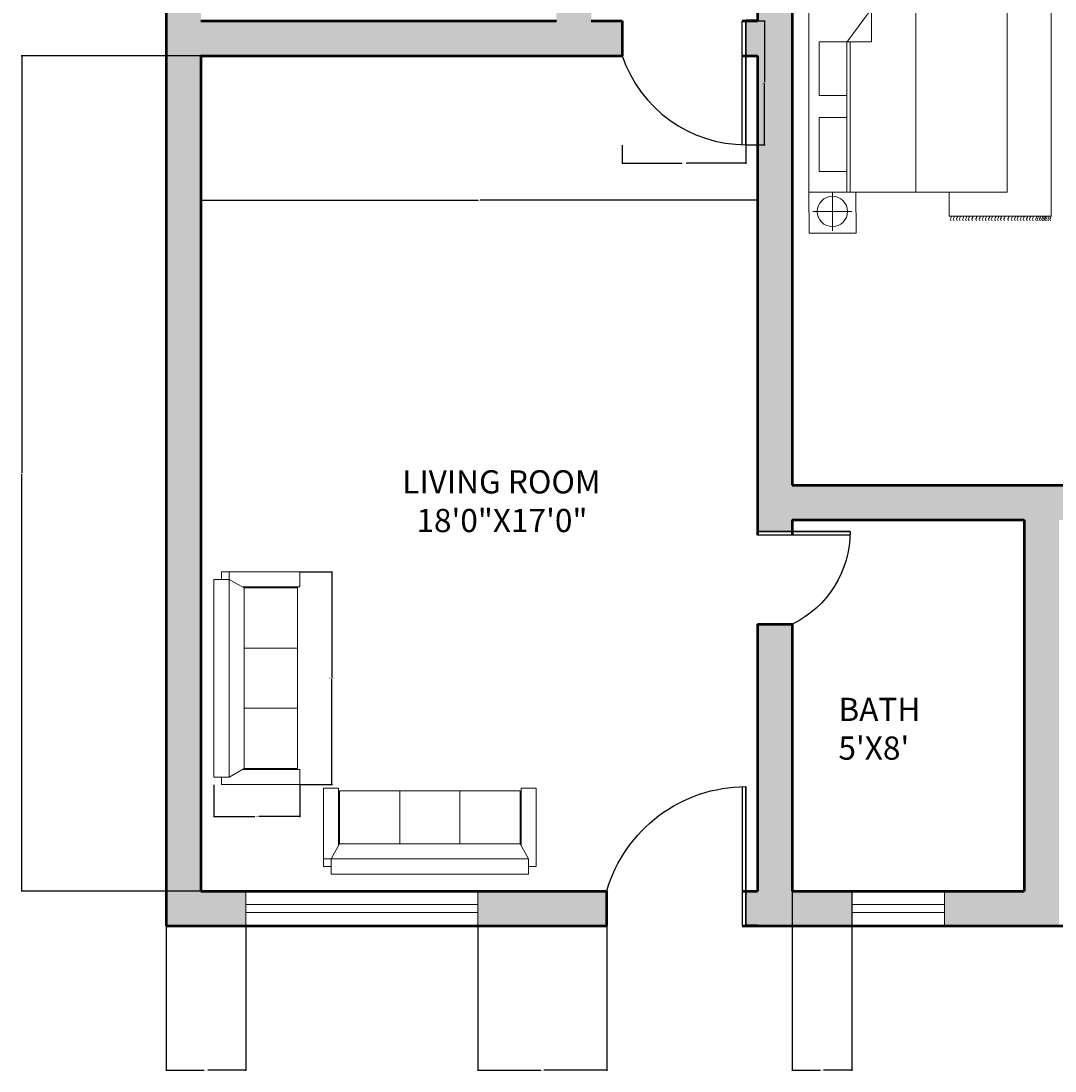
# Model space of a CAD drawing. Units: inches. Extents: x 383 to 970, y 275 to 1088.
# Tile 1 of 11: x 383 to 650, y 275 to 546. Entities that reach past the tile are written whole.
import ezdxf

# ---------------------------------------------------------------- set-up
doc = ezdxf.new("R2010")
doc.units = ezdxf.units.IN
doc.header["$MEASUREMENT"] = 0
for name, color, linetype, lineweight in [('A-ANNO-DIMS', 2, 'Continuous', 18), ('A-AREA-IDEN', 7, 'Continuous', 18), ('A-DOOR', 3, 'Continuous', 25), ('A-FURN', 8, 'Continuous', 18), ('A-GLAZ', 4, 'Continuous', 18), ('A-WALL', 7, 'Continuous', 50)]:
    doc.layers.add(name, color=color, linetype=linetype, lineweight=lineweight)
doc.layers.add('A-WALL-PATT', color=251, linetype='Continuous', lineweight=13, true_color=0x636466)
doc.styles.get("Standard").update_dxf_attribs({"font": 'arial.ttf'})
doc.dimstyles.get("Standard").update_dxf_attribs({"dimtxt": 0.18, "dimasz": 0.18, "dimexe": 0.18, "dimexo": 0.0625, "dimgap": 0.09, "dimtad": 0, "dimtih": 1, "dimtoh": 1, "dimdec": 4, "dimzin": 0, "dimdsep": 46, "dimtxsty": 'Standard', "dimcen": 0.09, "dimadec": 0, "dimazin": 0, "dimtfac": 1, "dimtdec": 4, "dimtofl": 0, "dimtmove": 0, "dimatfit": 3, "dimfxl": 1, "dimtolj": 1, "dimtzin": 0, "dimarcsym": 0})

# ---------------------------------------------------------------- blocks, each defined once
blk = doc.blocks.new('BED-DOUBLE-WITH-NIGHTSTANDS')
for p, q in [((6.09, 68.68), (6.09, 58.62)), ((36.42, 67.59), (62.78, 67.59)), ((36.42, 58.05), (36.42, 67.59)), ((62.78, 67.59), (62.78, 4.35)), ((1.07, 63.65), (11.12, 63.65)), ((9.97, 49.39), (16.32, 58)), ((16.32, 49.44), (16.32, 58)), ((27.82, 58.05), (27.82, 10.63)), ((9.97, 49.44), (16.32, 49.44)), ((9.97, 49.39), (9.97, 10.63)), ((10.78, 49.44), (10.78, 10.63)), ((6.2, 10.63), (6.2, 0.57)), ((36.42, 4.35), (36.42, 10.65)), ((1.17, 5.6), (11.22, 5.6)), ((62.78, 4.35), (36.42, 4.35))]:
    blk.add_line(p, q)
for points in [[(12.29, 58.05), (12.19, 68.68), (0, 68.68), (0.1, 58.05)], [(0.1, 58.05), (51.42, 58.05), (51.42, 10.63), (0.1, 10.63)], [(2.8, 49.44), (9.97, 49.44), (9.97, 35.55), (2.8, 35.55)], [(2.8, 29.88), (9.97, 29.88), (9.97, 15.98), (2.8, 15.98)], [(12.39, 0), (12.29, 10.63), (0.1, 10.63), (0.21, 0)]]:
    blk.add_lwpolyline(points, close=True)
for centre in [(6.09, 63.65), (6.2, 5.6)]:
    blk.add_circle(centre, 3.92)
for points, knots in [([(36.95, 68.71), (36.83, 68.61), (36.59, 68.42), (36.83, 68.08), (37, 67.8), (36.89, 67.65), (36.85, 67.58)], [0, 0, 0, 0, 0.400747, 0.791423, 1.067667, 1.29709, 1.29709, 1.29709, 1.29709]), ([(37.73, 68.71), (37.61, 68.61), (37.37, 68.42), (37.61, 68.08), (37.78, 67.8), (37.67, 67.65), (37.62, 67.58)], [0, 0, 0, 0, 0.400747, 0.791423, 1.067667, 1.29709, 1.29709, 1.29709, 1.29709]), ([(38.54, 68.71), (38.42, 68.61), (38.18, 68.42), (38.42, 68.08), (38.59, 67.8), (38.49, 67.65), (38.44, 67.58)], [0, 0, 0, 0, 0.400747, 0.791423, 1.067667, 1.29709, 1.29709, 1.29709, 1.29709]), ([(39.27, 68.71), (39.15, 68.61), (38.91, 68.42), (39.15, 68.08), (39.32, 67.8), (39.22, 67.65), (39.17, 67.58)], [0, 0, 0, 0, 0.400747, 0.791423, 1.067667, 1.29709, 1.29709, 1.29709, 1.29709]), ([(40.15, 68.71), (40.03, 68.61), (39.79, 68.42), (40.03, 68.08), (40.21, 67.8), (40.1, 67.65), (40.05, 67.58)], [0, 0, 0, 0, 0.400747, 0.791423, 1.067667, 1.29709, 1.29709, 1.29709, 1.29709]), ([(40.91, 68.71), (40.78, 68.61), (40.54, 68.42), (40.78, 68.08), (40.96, 67.8), (40.85, 67.65), (40.8, 67.58)], [0, 0, 0, 0, 0.400747, 0.791423, 1.067667, 1.29709, 1.29709, 1.29709, 1.29709]), ([(41.63, 68.71), (41.51, 68.61), (41.27, 68.42), (41.51, 68.08), (41.69, 67.8), (41.58, 67.65), (41.53, 67.58)], [0, 0, 0, 0, 0.400747, 0.791423, 1.067667, 1.29709, 1.29709, 1.29709, 1.29709]), ([(42.52, 68.71), (42.39, 68.61), (42.16, 68.42), (42.39, 68.08), (42.57, 67.8), (42.46, 67.65), (42.41, 67.58)], [0, 0, 0, 0, 0.400747, 0.791423, 1.067667, 1.29709, 1.29709, 1.29709, 1.29709]), ([(43.55, 68.71), (43.43, 68.61), (43.19, 68.42), (43.43, 68.08), (43.6, 67.8), (43.5, 67.65), (43.45, 67.58)], [0, 0, 0, 0, 0.400747, 0.791423, 1.067667, 1.29709, 1.29709, 1.29709, 1.29709]), ([(44.43, 68.71), (44.31, 68.61), (44.07, 68.42), (44.31, 68.08), (44.49, 67.8), (44.38, 67.65), (44.33, 67.58)], [0, 0, 0, 0, 0.400747, 0.791423, 1.067667, 1.29709, 1.29709, 1.29709, 1.29709]), ([(45.25, 68.71), (45.13, 68.61), (44.89, 68.42), (45.13, 68.08), (45.3, 67.8), (45.2, 67.65), (45.15, 67.58)], [0, 0, 0, 0, 0.400747, 0.791423, 1.067667, 1.29709, 1.29709, 1.29709, 1.29709]), ([(46.03, 68.71), (45.91, 68.61), (45.67, 68.42), (45.91, 68.08), (46.08, 67.8), (45.97, 67.65), (45.92, 67.58)], [0, 0, 0, 0, 0.400747, 0.791423, 1.067667, 1.29709, 1.29709, 1.29709, 1.29709]), ([(46.84, 68.71), (46.72, 68.61), (46.48, 68.42), (46.72, 68.08), (46.9, 67.8), (46.79, 67.65), (46.74, 67.58)], [0, 0, 0, 0, 0.400747, 0.791423, 1.067667, 1.29709, 1.29709, 1.29709, 1.29709]), ([(47.57, 68.71), (47.45, 68.61), (47.21, 68.42), (47.45, 68.08), (47.62, 67.8), (47.52, 67.65), (47.47, 67.58)], [0, 0, 0, 0, 0.400747, 0.791423, 1.067667, 1.29709, 1.29709, 1.29709, 1.29709]), ([(48.45, 68.71), (48.33, 68.61), (48.09, 68.42), (48.33, 68.08), (48.51, 67.8), (48.4, 67.65), (48.35, 67.58)], [0, 0, 0, 0, 0.400747, 0.791423, 1.067667, 1.29709, 1.29709, 1.29709, 1.29709]), ([(49.21, 68.71), (49.08, 68.61), (48.85, 68.42), (49.08, 68.08), (49.26, 67.8), (49.15, 67.65), (49.1, 67.58)], [0, 0, 0, 0, 0.400747, 0.791423, 1.067667, 1.29709, 1.29709, 1.29709, 1.29709]), ([(49.93, 68.71), (49.81, 68.61), (49.57, 68.42), (49.81, 68.08), (49.99, 67.8), (49.88, 67.65), (49.83, 67.58)], [0, 0, 0, 0, 0.400747, 0.791423, 1.067667, 1.29709, 1.29709, 1.29709, 1.29709]), ([(50.82, 68.71), (50.69, 68.61), (50.46, 68.42), (50.69, 68.08), (50.87, 67.8), (50.76, 67.65), (50.71, 67.58)], [0, 0, 0, 0, 0.400747, 0.791423, 1.067667, 1.29709, 1.29709, 1.29709, 1.29709]), ([(51.85, 68.71), (51.73, 68.61), (51.49, 68.42), (51.73, 68.08), (51.9, 67.8), (51.8, 67.65), (51.75, 67.58)], [0, 0, 0, 0, 0.400747, 0.791423, 1.067667, 1.29709, 1.29709, 1.29709, 1.29709]), ([(52.74, 68.71), (52.61, 68.61), (52.37, 68.42), (52.61, 68.08), (52.79, 67.8), (52.68, 67.65), (52.63, 67.58)], [0, 0, 0, 0, 0.400747, 0.791423, 1.067667, 1.29709, 1.29709, 1.29709, 1.29709]), ([(53.55, 68.71), (53.43, 68.61), (53.19, 68.42), (53.43, 68.08), (53.6, 67.8), (53.5, 67.65), (53.45, 67.58)], [0, 0, 0, 0, 0.400747, 0.791423, 1.067667, 1.29709, 1.29709, 1.29709, 1.29709]), ([(54.24, 68.71), (54.12, 68.61), (53.88, 68.42), (54.12, 68.08), (54.29, 67.8), (54.19, 67.65), (54.14, 67.58)], [0, 0, 0, 0, 0.400747, 0.791423, 1.067667, 1.29709, 1.29709, 1.29709, 1.29709]), ([(55.06, 68.71), (54.94, 68.61), (54.7, 68.42), (54.94, 68.08), (55.11, 67.8), (55, 67.65), (54.95, 67.58)], [0, 0, 0, 0, 0.400747, 0.791423, 1.067667, 1.29709, 1.29709, 1.29709, 1.29709]), ([(55.78, 68.71), (55.66, 68.61), (55.42, 68.42), (55.66, 68.08), (55.84, 67.8), (55.73, 67.65), (55.68, 67.58)], [0, 0, 0, 0, 0.400747, 0.791423, 1.067667, 1.29709, 1.29709, 1.29709, 1.29709]), ([(56.67, 68.71), (56.55, 68.61), (56.31, 68.42), (56.55, 68.08), (56.72, 67.8), (56.61, 67.65), (56.56, 67.58)], [0, 0, 0, 0, 0.400747, 0.791423, 1.067667, 1.29709, 1.29709, 1.29709, 1.29709]), ([(57.42, 68.71), (57.3, 68.61), (57.06, 68.42), (57.3, 68.08), (57.47, 67.8), (57.36, 67.65), (57.32, 67.58)], [0, 0, 0, 0, 0.400747, 0.791423, 1.067667, 1.29709, 1.29709, 1.29709, 1.29709]), ([(58.15, 68.71), (58.03, 68.61), (57.79, 68.42), (58.03, 68.08), (58.2, 67.8), (58.1, 67.66), (58.05, 67.59)], [0, 0, 0, 0, 0.400747, 0.791423, 1.067667, 1.283686, 1.283686, 1.283686, 1.283686]), ([(59.03, 68.71), (58.91, 68.61), (58.67, 68.42), (58.91, 68.08), (59.08, 67.8), (58.98, 67.66), (58.93, 67.59)], [0, 0, 0, 0, 0.400747, 0.791423, 1.067667, 1.283686, 1.283686, 1.283686, 1.283686]), ([(59.46, 68.71), (59.34, 68.61), (59.09, 68.42), (59.34, 68.08), (59.51, 67.8), (59.41, 67.66), (59.36, 67.59)], [0, 0, 0, 0, 0.402903, 0.794912, 1.071156, 1.287177, 1.287177, 1.287177, 1.287177]), ([(60.05, 68.71), (59.93, 68.61), (59.69, 68.42), (59.93, 68.08), (60.1, 67.8), (60, 67.66), (59.96, 67.59)], [0, 0, 0, 0, 0.400747, 0.791423, 1.067667, 1.283686, 1.283686, 1.283686, 1.283686]), ([(60.63, 68.71), (60.51, 68.61), (60.27, 68.42), (60.51, 68.08), (60.68, 67.8), (60.58, 67.66), (60.53, 67.59)], [0, 0, 0, 0, 0.400747, 0.791423, 1.067667, 1.283686, 1.283686, 1.283686, 1.283686]), ([(60.94, 68.71), (60.82, 68.61), (60.58, 68.42), (60.81, 68.08), (60.99, 67.8), (60.89, 67.66), (60.84, 67.59)], [0, 0, 0, 0, 0.400747, 0.791423, 1.067667, 1.283686, 1.283686, 1.283686, 1.283686]), ([(61.36, 68.71), (61.23, 68.61), (60.99, 68.42), (61.23, 68.08), (61.41, 67.8), (61.3, 67.65), (61.25, 67.58)], [0, 0, 0, 0, 0.400747, 0.791423, 1.067667, 1.29709, 1.29709, 1.29709, 1.29709]), ([(61.75, 68.71), (61.63, 68.61), (61.39, 68.42), (61.63, 68.08), (61.8, 67.8), (61.7, 67.65), (61.65, 67.58)], [0, 0, 0, 0, 0.400747, 0.791423, 1.067667, 1.29709, 1.29709, 1.29709, 1.29709]), ([(62.24, 68.71), (62.12, 68.61), (61.88, 68.42), (62.12, 68.08), (62.29, 67.8), (62.18, 67.65), (62.13, 67.58)], [0, 0, 0, 0, 0.400747, 0.791423, 1.067667, 1.29709, 1.29709, 1.29709, 1.29709]), ([(62.71, 68.71), (62.59, 68.61), (62.35, 68.42), (62.59, 68.08), (62.76, 67.8), (62.66, 67.65), (62.61, 67.58)], [0, 0, 0, 0, 0.400747, 0.791423, 1.067667, 1.29709, 1.29709, 1.29709, 1.29709]), ([(36.95, 3.23), (36.83, 3.32), (36.59, 3.52), (36.83, 3.86), (37, 4.14), (36.89, 4.29), (36.85, 4.35)], [0, 0, 0, 0, 0.400747, 0.791423, 1.067667, 1.29709, 1.29709, 1.29709, 1.29709]), ([(37.73, 3.23), (37.61, 3.32), (37.37, 3.52), (37.61, 3.86), (37.78, 4.14), (37.67, 4.29), (37.62, 4.35)], [0, 0, 0, 0, 0.400747, 0.791423, 1.067667, 1.29709, 1.29709, 1.29709, 1.29709]), ([(38.54, 3.23), (38.42, 3.32), (38.18, 3.52), (38.42, 3.86), (38.59, 4.14), (38.49, 4.29), (38.44, 4.35)], [0, 0, 0, 0, 0.400747, 0.791423, 1.067667, 1.29709, 1.29709, 1.29709, 1.29709]), ([(39.27, 3.23), (39.15, 3.32), (38.91, 3.52), (39.15, 3.86), (39.32, 4.14), (39.22, 4.29), (39.17, 4.35)], [0, 0, 0, 0, 0.400747, 0.791423, 1.067667, 1.29709, 1.29709, 1.29709, 1.29709]), ([(40.15, 3.23), (40.03, 3.32), (39.79, 3.52), (40.03, 3.86), (40.21, 4.14), (40.1, 4.29), (40.05, 4.35)], [0, 0, 0, 0, 0.400747, 0.791423, 1.067667, 1.29709, 1.29709, 1.29709, 1.29709]), ([(40.91, 3.23), (40.78, 3.32), (40.54, 3.52), (40.78, 3.86), (40.96, 4.14), (40.85, 4.29), (40.8, 4.35)], [0, 0, 0, 0, 0.400747, 0.791423, 1.067667, 1.29709, 1.29709, 1.29709, 1.29709]), ([(41.63, 3.23), (41.51, 3.32), (41.27, 3.52), (41.51, 3.86), (41.69, 4.14), (41.58, 4.29), (41.53, 4.35)], [0, 0, 0, 0, 0.400747, 0.791423, 1.067667, 1.29709, 1.29709, 1.29709, 1.29709]), ([(42.52, 3.23), (42.39, 3.32), (42.16, 3.52), (42.39, 3.86), (42.57, 4.14), (42.46, 4.29), (42.41, 4.35)], [0, 0, 0, 0, 0.400747, 0.791423, 1.067667, 1.29709, 1.29709, 1.29709, 1.29709]), ([(43.55, 3.23), (43.43, 3.32), (43.19, 3.52), (43.43, 3.86), (43.6, 4.14), (43.5, 4.29), (43.45, 4.35)], [0, 0, 0, 0, 0.400747, 0.791423, 1.067667, 1.29709, 1.29709, 1.29709, 1.29709]), ([(44.43, 3.23), (44.31, 3.32), (44.07, 3.52), (44.31, 3.86), (44.49, 4.14), (44.38, 4.29), (44.33, 4.35)], [0, 0, 0, 0, 0.400747, 0.791423, 1.067667, 1.29709, 1.29709, 1.29709, 1.29709]), ([(45.25, 3.23), (45.13, 3.32), (44.89, 3.52), (45.13, 3.86), (45.3, 4.14), (45.2, 4.29), (45.15, 4.35)], [0, 0, 0, 0, 0.400747, 0.791423, 1.067667, 1.29709, 1.29709, 1.29709, 1.29709]), ([(46.03, 3.23), (45.91, 3.32), (45.67, 3.52), (45.91, 3.86), (46.08, 4.14), (45.97, 4.29), (45.92, 4.35)], [0, 0, 0, 0, 0.400747, 0.791423, 1.067667, 1.29709, 1.29709, 1.29709, 1.29709]), ([(46.84, 3.23), (46.72, 3.32), (46.48, 3.52), (46.72, 3.86), (46.9, 4.14), (46.79, 4.29), (46.74, 4.35)], [0, 0, 0, 0, 0.400747, 0.791423, 1.067667, 1.29709, 1.29709, 1.29709, 1.29709]), ([(47.57, 3.23), (47.45, 3.32), (47.21, 3.52), (47.45, 3.86), (47.62, 4.14), (47.52, 4.29), (47.47, 4.35)], [0, 0, 0, 0, 0.400747, 0.791423, 1.067667, 1.29709, 1.29709, 1.29709, 1.29709]), ([(48.45, 3.23), (48.33, 3.32), (48.09, 3.52), (48.33, 3.86), (48.51, 4.14), (48.4, 4.29), (48.35, 4.35)], [0, 0, 0, 0, 0.400747, 0.791423, 1.067667, 1.29709, 1.29709, 1.29709, 1.29709]), ([(49.21, 3.23), (49.08, 3.32), (48.85, 3.52), (49.08, 3.86), (49.26, 4.14), (49.15, 4.29), (49.1, 4.35)], [0, 0, 0, 0, 0.400747, 0.791423, 1.067667, 1.29709, 1.29709, 1.29709, 1.29709]), ([(49.93, 3.23), (49.81, 3.32), (49.57, 3.52), (49.81, 3.86), (49.99, 4.14), (49.88, 4.29), (49.83, 4.35)], [0, 0, 0, 0, 0.400747, 0.791423, 1.067667, 1.29709, 1.29709, 1.29709, 1.29709]), ([(50.82, 3.23), (50.69, 3.32), (50.46, 3.52), (50.69, 3.86), (50.87, 4.14), (50.76, 4.29), (50.71, 4.35)], [0, 0, 0, 0, 0.400747, 0.791423, 1.067667, 1.29709, 1.29709, 1.29709, 1.29709]), ([(51.85, 3.23), (51.73, 3.32), (51.49, 3.52), (51.73, 3.86), (51.9, 4.14), (51.8, 4.29), (51.75, 4.35)], [0, 0, 0, 0, 0.400747, 0.791423, 1.067667, 1.29709, 1.29709, 1.29709, 1.29709]), ([(52.74, 3.23), (52.61, 3.32), (52.37, 3.52), (52.61, 3.86), (52.79, 4.14), (52.68, 4.29), (52.63, 4.35)], [0, 0, 0, 0, 0.400747, 0.791423, 1.067667, 1.29709, 1.29709, 1.29709, 1.29709]), ([(53.55, 3.23), (53.43, 3.32), (53.19, 3.52), (53.43, 3.86), (53.6, 4.14), (53.5, 4.29), (53.45, 4.35)], [0, 0, 0, 0, 0.400747, 0.791423, 1.067667, 1.29709, 1.29709, 1.29709, 1.29709]), ([(54.24, 3.23), (54.12, 3.32), (53.88, 3.52), (54.12, 3.86), (54.29, 4.14), (54.19, 4.29), (54.14, 4.35)], [0, 0, 0, 0, 0.400747, 0.791423, 1.067667, 1.29709, 1.29709, 1.29709, 1.29709]), ([(55.06, 3.23), (54.94, 3.32), (54.7, 3.52), (54.94, 3.86), (55.11, 4.14), (55, 4.29), (54.95, 4.35)], [0, 0, 0, 0, 0.400747, 0.791423, 1.067667, 1.29709, 1.29709, 1.29709, 1.29709]), ([(55.78, 3.23), (55.66, 3.32), (55.42, 3.52), (55.66, 3.86), (55.84, 4.14), (55.73, 4.29), (55.68, 4.35)], [0, 0, 0, 0, 0.400747, 0.791423, 1.067667, 1.29709, 1.29709, 1.29709, 1.29709]), ([(56.67, 3.23), (56.55, 3.32), (56.31, 3.52), (56.55, 3.86), (56.72, 4.14), (56.61, 4.29), (56.56, 4.35)], [0, 0, 0, 0, 0.400747, 0.791423, 1.067667, 1.29709, 1.29709, 1.29709, 1.29709]), ([(57.42, 3.23), (57.3, 3.32), (57.06, 3.52), (57.3, 3.86), (57.47, 4.14), (57.36, 4.29), (57.32, 4.35)], [0, 0, 0, 0, 0.400747, 0.791423, 1.067667, 1.29709, 1.29709, 1.29709, 1.29709]), ([(58.15, 3.23), (58.03, 3.32), (57.79, 3.52), (58.03, 3.86), (58.2, 4.14), (58.09, 4.29), (58.04, 4.35)], [0, 0, 0, 0, 0.400747, 0.791423, 1.067667, 1.29709, 1.29709, 1.29709, 1.29709]), ([(59.03, 3.23), (58.91, 3.32), (58.67, 3.52), (58.91, 3.86), (59.08, 4.14), (58.98, 4.29), (58.93, 4.35)], [0, 0, 0, 0, 0.400747, 0.791423, 1.067667, 1.29709, 1.29709, 1.29709, 1.29709]), ([(59.46, 3.23), (59.33, 3.32), (59.08, 3.52), (59.34, 3.86), (59.51, 4.14), (59.4, 4.29), (59.36, 4.35)], [0, 0, 0, 0, 0.407265, 0.802015, 1.07826, 1.307683, 1.307683, 1.307683, 1.307683]), ([(60.03, 3.23), (59.9, 3.32), (59.67, 3.52), (59.9, 3.86), (60.08, 4.14), (59.97, 4.29), (59.92, 4.35)], [0, 0, 0, 0, 0.400747, 0.791423, 1.067667, 1.29709, 1.29709, 1.29709, 1.29709]), ([(60.6, 3.23), (60.48, 3.32), (60.24, 3.52), (60.48, 3.86), (60.65, 4.14), (60.54, 4.29), (60.5, 4.35)], [0, 0, 0, 0, 0.400747, 0.791423, 1.067667, 1.29709, 1.29709, 1.29709, 1.29709]), ([(60.91, 3.23), (60.79, 3.32), (60.55, 3.52), (60.79, 3.86), (60.96, 4.14), (60.85, 4.29), (60.81, 4.35)], [0, 0, 0, 0, 0.400747, 0.791423, 1.067667, 1.29709, 1.29709, 1.29709, 1.29709]), ([(61.33, 3.23), (61.21, 3.32), (60.97, 3.52), (61.21, 3.86), (61.38, 4.14), (61.27, 4.29), (61.22, 4.35)], [0, 0, 0, 0, 0.400747, 0.791423, 1.067667, 1.29709, 1.29709, 1.29709, 1.29709]), ([(61.72, 3.23), (61.6, 3.32), (61.36, 3.52), (61.6, 3.86), (61.78, 4.14), (61.67, 4.29), (61.62, 4.35)], [0, 0, 0, 0, 0.400747, 0.791423, 1.067667, 1.29709, 1.29709, 1.29709, 1.29709]), ([(62.21, 3.23), (62.09, 3.32), (61.85, 3.52), (62.09, 3.86), (62.26, 4.14), (62.16, 4.29), (62.11, 4.35)], [0, 0, 0, 0, 0.400747, 0.791423, 1.067667, 1.29709, 1.29709, 1.29709, 1.29709]), ([(62.71, 3.23), (62.59, 3.32), (62.35, 3.52), (62.59, 3.86), (62.76, 4.14), (62.66, 4.29), (62.61, 4.35)], [0, 0, 0, 0, 0.400747, 0.791423, 1.067667, 1.29709, 1.29709, 1.29709, 1.29709])]:
    blk.add_open_spline(points, degree=3, knots=knots)
blk = doc.blocks.new('SOFA-3-SEAT')
for p, q in [((1.96, 55.04), (22.23, 55.04)), ((1.96, 55.04), (1.96, 53.08)), ((3.92, 55.04), (3.92, 1.96)), ((22.23, 51.12), (22.23, 55.04)), ((0, 53.08), (0, 1.96)), ((3.92, 53.08), (0, 53.08)), ((3.92, 53.08), (7.85, 50.88)), ((7.54, 51.12), (22.23, 51.12)), ((21.58, 50.87), (7.85, 50.87)), ((21.58, 35.3), (7.85, 35.3)), ((21.58, 19.74), (7.85, 19.74)), ((7.85, 4.17), (3.92, 1.96)), ((7.29, 3.92), (22.23, 3.92)), ((22.23, 3.92), (22.23, 0)), ((3.92, 1.96), (0, 1.96)), ((1.96, 1.96), (1.96, 0)), ((1.96, 0), (22.23, 0))]:
    blk.add_line(p, q)
blk.add_lwpolyline([(7.85, 50.88), (7.85, 4.17), (21.58, 4.17), (21.58, 50.87)])
blk = doc.blocks.new('DOOR-LEAF-36IN')
for p, q in [((0, 0), (0, 36)), ((1, 36), (1, 0)), ((0, 0), (1, 0))]:
    blk.add_line(p, q)
blk.add_arc((0, -1.5), 37.5, 16.2602, 90)
blk = doc.blocks.new('DOOR-LEAF-24IN')
for p, q in [((23, 24), (23, 0)), ((24, 0), (24, 24)), ((24, 0), (23, 0))]:
    blk.add_line(p, q)
blk.add_arc((24, -2.7), 26.7, 90, 154.0108)
blk = doc.blocks.new('WIN-VENT-24IN')
for p, q in [((0, 0), (0, 24)), ((3.5, 0), (3.5, 24)), ((5.5, 24), (5.5, 0)), ((9, 24), (9, 0))]:
    blk.add_line(p, q)
blk = doc.blocks.new('WIN-60IN')
for p, q in [((60, 9), (0, 9)), ((60, 5.5), (0, 5.5)), ((0, 3.5), (60, 3.5)), ((0, 0), (60, 0))]:
    blk.add_line(p, q)
blk = doc.blocks.new('DOOR-LEAF-32IN')
for p, q in [((32, 32), (31, 32)), ((31, 0), (31, 32)), ((32, 32), (32, 0))]:
    blk.add_line(p, q)
blk.add_arc((32, 33.76), 33.76, 198.5866, 270)
blk = doc.blocks.new('*D15')
at = {"layer": 'A-ANNO-DIMS', "color": 0, "lineweight": -2, "transparency": 16777216}
for p, q in [((570.3, 546.14), (575.22, 546.14)), ((575.04, 545.96), (575.04, 530.32)), ((575.04, 514.32), (575.04, 529.95)), ((570.3, 514.14), (575.22, 514.14))]:
    blk.add_line(p, q, dxfattribs=at)
at = {"layer": 'A-ANNO-DIMS', "color": 0, "transparency": 16777216}
for points in [[(575.01, 545.96), (575.07, 545.96), (575.04, 546.14)], [(575.01, 514.32), (575.07, 514.32), (575.04, 514.14)]]:
    blk.add_solid(points, dxfattribs=at)
at = {"layer": 'Defpoints', "color": 0, "transparency": 16777216}
for p in [(570.24, 546.14), (575.04, 546.14), (570.24, 514.14)]:
    blk.add_point(p, dxfattribs=at)
at = {"layer": 'A-ANNO-DIMS', "color": 0, "transparency": 16777216, "insert": (575.04, 530.14), "char_height": 0.18, "attachment_point": 5}
blk.add_mtext('\\A1;D2 32 TYP.', dxfattribs=at)
blk = doc.blocks.new('*D16')
at = {"layer": 'A-ANNO-DIMS', "color": 0, "lineweight": -2, "transparency": 16777216}
for p, q in [((538.24, 514.07), (538.24, 509.16)), ((570.24, 514.07), (570.24, 509.16)), ((538.42, 509.34), (553.71, 509.34)), ((570.06, 509.34), (554.77, 509.34))]:
    blk.add_line(p, q, dxfattribs=at)
at = {"layer": 'A-ANNO-DIMS', "color": 0, "transparency": 16777216}
for points in [[(538.42, 509.37), (538.42, 509.31), (538.24, 509.34)], [(570.06, 509.37), (570.06, 509.31), (570.24, 509.34)]]:
    blk.add_solid(points, dxfattribs=at)
at = {"layer": 'Defpoints', "color": 0, "transparency": 16777216}
for p in [(538.24, 514.14), (570.24, 514.14), (570.24, 509.34)]:
    blk.add_point(p, dxfattribs=at)
at = {"layer": 'A-ANNO-DIMS', "color": 0, "transparency": 16777216, "insert": (554.24, 509.34), "char_height": 0.18, "attachment_point": 5}
blk.add_mtext('\\A1;32 TYP.', dxfattribs=at)
blk = doc.blocks.new('*D29')
at = {"layer": 'A-ANNO-DIMS', "color": 0, "lineweight": -2, "transparency": 16777216}
for p, q in [((454.91, 403.71), (463.28, 403.71)), ((463.1, 403.53), (463.1, 376.37)), ((463.1, 348.85), (463.1, 376.01)), ((454.91, 348.67), (463.28, 348.67))]:
    blk.add_line(p, q, dxfattribs=at)
at = {"layer": 'A-ANNO-DIMS', "color": 0, "transparency": 16777216}
for points in [[(463.07, 403.53), (463.13, 403.53), (463.1, 403.71)], [(463.07, 348.85), (463.13, 348.85), (463.1, 348.67)]]:
    blk.add_solid(points, dxfattribs=at)
at = {"layer": 'Defpoints', "color": 0, "transparency": 16777216}
for p in [(454.85, 403.71), (463.1, 403.71), (454.85, 348.67)]:
    blk.add_point(p, dxfattribs=at)
at = {"layer": 'A-ANNO-DIMS', "color": 0, "transparency": 16777216, "insert": (463.1, 376.19), "char_height": 0.18, "attachment_point": 5}
blk.add_mtext('\\A1;SOFA 55 TYP.', dxfattribs=at)
blk = doc.blocks.new('*D30')
at = {"layer": 'A-ANNO-DIMS', "color": 0, "lineweight": -2, "transparency": 16777216}
for p, q in [((432.62, 348.61), (432.62, 340.23)), ((454.85, 348.61), (454.85, 340.23)), ((432.8, 340.41), (443.2, 340.41)), ((454.67, 340.41), (444.26, 340.41))]:
    blk.add_line(p, q, dxfattribs=at)
at = {"layer": 'A-ANNO-DIMS', "color": 0, "transparency": 16777216}
for points in [[(432.8, 340.44), (432.8, 340.38), (432.62, 340.41)], [(454.67, 340.44), (454.67, 340.38), (454.85, 340.41)]]:
    blk.add_solid(points, dxfattribs=at)
at = {"layer": 'Defpoints', "color": 0, "transparency": 16777216}
for p in [(432.62, 348.67), (454.85, 348.67), (454.85, 340.41)]:
    blk.add_point(p, dxfattribs=at)
at = {"layer": 'A-ANNO-DIMS', "color": 0, "transparency": 16777216, "insert": (443.73, 340.41), "char_height": 0.18, "attachment_point": 5}
blk.add_mtext('\\A1;22 TYP.', dxfattribs=at)
blk = doc.blocks.new('*D40')
at = {"layer": 'A-ANNO-DIMS', "color": 0, "lineweight": -2, "transparency": 16777216}
for p, q in [((429.18, 537.14), (382.71, 537.14)), ((382.89, 536.96), (382.89, 429.32)), ((382.89, 321.32), (382.89, 428.95)), ((429.18, 321.14), (382.71, 321.14))]:
    blk.add_line(p, q, dxfattribs=at)
at = {"layer": 'A-ANNO-DIMS', "color": 0, "transparency": 16777216}
for points in [[(382.86, 536.96), (382.92, 536.96), (382.89, 537.14)], [(382.86, 321.32), (382.92, 321.32), (382.89, 321.14)]]:
    blk.add_solid(points, dxfattribs=at)
at = {"layer": 'Defpoints', "color": 0, "transparency": 16777216}
for p in [(382.89, 537.14), (429.24, 537.14), (429.24, 321.14)]:
    blk.add_point(p, dxfattribs=at)
at = {"layer": 'A-ANNO-DIMS', "color": 0, "transparency": 16777216, "insert": (382.89, 429.14), "char_height": 0.18, "attachment_point": 5}
blk.add_mtext('\\A1;216', dxfattribs=at)
blk = doc.blocks.new('*D41')
at = {"layer": 'A-ANNO-DIMS', "color": 0, "lineweight": -2, "transparency": 16777216}
for p, q in [((429.24, 537.07), (429.24, 499.61)), ((573.24, 537.07), (573.24, 499.61)), ((429.42, 499.79), (500.96, 499.79)), ((573.06, 499.79), (501.52, 499.79))]:
    blk.add_line(p, q, dxfattribs=at)
at = {"layer": 'A-ANNO-DIMS', "color": 0, "transparency": 16777216}
for points in [[(429.42, 499.82), (429.42, 499.76), (429.24, 499.79)], [(573.06, 499.82), (573.06, 499.76), (573.24, 499.79)]]:
    blk.add_solid(points, dxfattribs=at)
at = {"layer": 'Defpoints', "color": 0, "transparency": 16777216}
for p in [(429.24, 537.14), (573.24, 537.14), (429.24, 499.79)]:
    blk.add_point(p, dxfattribs=at)
at = {"layer": 'A-ANNO-DIMS', "color": 0, "transparency": 16777216, "insert": (501.24, 499.79), "char_height": 0.18, "attachment_point": 5}
blk.add_mtext('\\A1;144', dxfattribs=at)
blk = doc.blocks.new('*D50')
at = {"layer": 'A-ANNO-DIMS', "color": 0, "lineweight": -2, "transparency": 16777216}
for p, q in [((420.24, 312.07), (420.24, 274.61)), ((440.89, 312.07), (440.89, 274.61)), ((420.42, 274.79), (430.1, 274.79)), ((440.71, 274.79), (431.03, 274.79))]:
    blk.add_line(p, q, dxfattribs=at)
at = {"layer": 'A-ANNO-DIMS', "color": 0, "transparency": 16777216}
for points in [[(420.42, 274.82), (420.42, 274.76), (420.24, 274.79)], [(440.71, 274.82), (440.71, 274.76), (440.89, 274.79)]]:
    blk.add_solid(points, dxfattribs=at)
at = {"layer": 'Defpoints', "color": 0, "transparency": 16777216}
for p in [(420.24, 312.14), (440.89, 312.14), (440.89, 274.79)]:
    blk.add_point(p, dxfattribs=at)
at = {"layer": 'A-ANNO-DIMS', "color": 0, "transparency": 16777216, "insert": (430.56, 274.79), "char_height": 0.18, "attachment_point": 5}
blk.add_mtext('\\A1;20.647', dxfattribs=at)
blk = doc.blocks.new('*D51')
at = {"layer": 'A-ANNO-DIMS', "color": 0, "lineweight": -2, "transparency": 16777216}
for p, q in [((500.89, 312.07), (500.89, 274.61)), ((534.24, 312.07), (534.24, 274.61)), ((501.07, 274.79), (517.17, 274.79)), ((534.06, 274.79), (517.96, 274.79))]:
    blk.add_line(p, q, dxfattribs=at)
at = {"layer": 'A-ANNO-DIMS', "color": 0, "transparency": 16777216}
for points in [[(501.07, 274.82), (501.07, 274.76), (500.89, 274.79)], [(534.06, 274.82), (534.06, 274.76), (534.24, 274.79)]]:
    blk.add_solid(points, dxfattribs=at)
at = {"layer": 'Defpoints', "color": 0, "transparency": 16777216}
for p in [(500.89, 312.14), (534.24, 312.14), (534.24, 274.79)]:
    blk.add_point(p, dxfattribs=at)
at = {"layer": 'A-ANNO-DIMS', "color": 0, "transparency": 16777216, "insert": (517.56, 274.79), "char_height": 0.18, "attachment_point": 5}
blk.add_mtext('\\A1;33.35', dxfattribs=at)
blk = doc.blocks.new('*D66')
at = {"layer": 'A-ANNO-DIMS', "color": 0, "lineweight": -2, "transparency": 16777216}
for p, q in [((582.24, 321.07), (582.24, 274.61)), ((597.62, 321.07), (597.62, 274.61)), ((582.42, 274.79), (589.54, 274.79)), ((597.44, 274.79), (590.32, 274.79))]:
    blk.add_line(p, q, dxfattribs=at)
at = {"layer": 'A-ANNO-DIMS', "color": 0, "transparency": 16777216}
for points in [[(582.42, 274.82), (582.42, 274.76), (582.24, 274.79)], [(597.44, 274.82), (597.44, 274.76), (597.62, 274.79)]]:
    blk.add_solid(points, dxfattribs=at)
at = {"layer": 'Defpoints', "color": 0, "transparency": 16777216}
for p in [(582.24, 321.14), (597.62, 321.14), (597.62, 274.79)]:
    blk.add_point(p, dxfattribs=at)
at = {"layer": 'A-ANNO-DIMS', "color": 0, "transparency": 16777216, "insert": (589.93, 274.79), "char_height": 0.18, "attachment_point": 5}
blk.add_mtext('\\A1;15.38', dxfattribs=at)

msp = doc.modelspace()

# ---------------------------------------------------------------- hatches: boundary and pattern name
at = {"layer": 'A-WALL-PATT'}
h = msp.add_hatch(color=256, dxfattribs=at)
h.dxf.hatch_style = 1
h.paths.add_polyline_path([(651.24, 321.1365), (651.24, 417.1365), (735.24, 417.1365), (735.24, 491.9233), (726.24, 491.9233), (726.24, 426.1365), (582.24, 426.1365), (582.24, 606.1365), (687.24, 606.1365), (687.24, 615.1365), (573.24, 615.1365), (573.24, 546.1365), (570.24, 546.1365), (570.24, 537.1365), (573.24, 537.1365), (573.24, 414.1365), (582.24, 414.1365), (582.24, 417.1365), (642.24, 417.1365), (642.24, 321.1365), (621.6203, 321.1365), (621.6203, 312.1365), (651.24, 312.1365)], flags=17)
h.paths.add_polyline_path([(597.6203, 321.1365), (582.24, 321.1365), (582.24, 390.1365), (573.24, 390.1365), (573.24, 321.1365), (570.24, 321.1365), (570.24, 312.1365), (573.24, 312.1365), (597.6203, 312.1365)], flags=16)
h.paths.add_polyline_path([(534.24, 321.1365), (500.8868, 321.1365), (500.8868, 312.1365), (534.24, 312.1365)], flags=17)
h.paths.add_polyline_path([(735.24, 606.1365), (738.24, 606.1365), (738.24, 615.1365), (723.24, 615.1365), (723.24, 606.1365), (726.24, 606.1365), (726.24, 551.9233), (735.24, 551.9233)], flags=17)
h.paths.add_polyline_path([(848.0899, 615.1365), (814.24, 615.1365), (814.24, 689.38), (805.24, 689.38), (805.24, 615.1365), (802.24, 615.1365), (802.24, 606.1365), (848.0899, 606.1365)], flags=17)
h.paths.add_polyline_path([(530.24, 615.1365), (498.24, 615.1365), (498.24, 646.5351), (489.24, 646.5351), (489.24, 615.1365), (466.771, 615.1365), (466.771, 606.1365), (521.24, 606.1365), (521.24, 603.1365), (530.24, 603.1365), (530.24, 606.1365)], flags=17)
h.paths.add_polyline_path([(498.24, 744.1365), (489.24, 744.1365), (489.24, 706.5351), (498.24, 706.5351)], flags=17)
h.paths.add_polyline_path([(715.24, 792.1365), (598.24, 792.1365), (598.24, 972.1365), (636.5058, 972.1365), (636.5058, 981.1365), (589.24, 981.1365), (589.24, 972.1365), (589.24, 792.1365), (586.24, 792.1365), (586.24, 783.1365), (589.24, 783.1365), (715.24, 783.1365)], flags=17)
h.paths.add_polyline_path([(763.24, 981.1365), (696.5058, 981.1365), (696.5058, 972.1365), (754.24, 972.1365), (754.24, 792.1365), (751.24, 792.1365), (751.24, 783.1365), (754.24, 783.1365), (764.24, 783.1365), (764.24, 792.1365), (763.24, 792.1365)], flags=17)
h.paths.add_polyline_path([(815.24, 1001.9492), (806.24, 1001.9492), (806.24, 972.1365), (818.24, 972.1365), (818.24, 981.1365), (815.24, 981.1365)], flags=17)
h.paths.add_polyline_path([(546.24, 1004.0336), (537.24, 1004.0336), (537.24, 981.1365), (534.24, 981.1365), (534.24, 972.1365), (537.24, 972.1365), (546.24, 972.1365), (546.24, 981.1365)], flags=17)
h.paths.add_polyline_path([(884.0899, 606.1365), (932.24, 606.1365), (932.24, 1050.1365), (420.24, 1050.1365), (420.24, 312.1365), (440.8868, 312.1365), (440.8868, 321.1365), (429.24, 321.1365), (429.24, 537.1365), (538.24, 537.1365), (538.24, 546.1365), (530.24, 546.1365), (530.24, 579.1365), (521.24, 579.1365), (521.24, 546.1365), (429.24, 546.1365), (429.24, 606.1365), (442.771, 606.1365), (442.771, 615.1365), (429.24, 615.1365), (429.24, 783.1365), (489.24, 783.1365), (489.24, 780.1365), (498.24, 780.1365), (498.24, 783.1365), (550.24, 783.1365), (550.24, 792.1365), (429.24, 792.1365), (429.24, 972.1365), (510.24, 972.1365), (510.24, 981.1365), (429.24, 981.1365), (429.24, 1041.1365), (537.24, 1041.1365), (537.24, 1028.0336), (546.24, 1028.0336), (546.24, 1041.1365), (806.24, 1041.1365), (806.24, 1025.9492), (815.24, 1025.9492), (815.24, 1041.1365), (923.24, 1041.1365), (923.24, 981.1365), (842.24, 981.1365), (842.24, 972.1365), (923.24, 972.1365), (923.24, 792.1365), (800.24, 792.1365), (800.24, 783.1365), (805.24, 783.1365), (805.24, 725.38), (814.24, 725.38), (814.24, 783.1365), (923.24, 783.1365), (923.24, 615.1365), (884.0899, 615.1365)])

# ---------------------------------------------------------------- linework, layer by layer
at = {"layer": 'A-DOOR'}
for p, q in [((570.24, 514.1365), (570.24, 546.1365)), ((597.24, 414.1365), (573.24, 414.1365)), ((570.24, 348.1365), (570.24, 312.1365))]:
    msp.add_line(p, q, dxfattribs=at)
at = {"layer": 'A-GLAZ'}
for p, q in [((440.8868, 321.1365), (440.8868, 312.1365)), ((500.8868, 312.1365), (500.8868, 321.1365)), ((597.6203, 321.1365), (597.6203, 312.1365)), ((621.6203, 312.1365), (621.6203, 321.1365))]:
    msp.add_line(p, q, dxfattribs=at)
at = {"layer": 'A-WALL'}
for p, q in [((420.24, 1050.1365), (420.24, 312.1365)), ((573.24, 615.1365), (573.24, 546.1365)), ((582.24, 606.1365), (582.24, 426.1365)), ((429.24, 546.1365), (521.24, 546.1365)), ((530.24, 546.1365), (538.24, 546.1365)), ((538.24, 546.1365), (538.24, 537.1365)), ((569.24, 546.1365), (573.24, 546.1365)), ((573.24, 546.1365), (570.24, 546.1365)), ((429.24, 537.1365), (538.24, 537.1365)), ((429.24, 537.1365), (429.24, 321.1365)), ((569.24, 537.1365), (573.24, 537.1365)), ((573.24, 537.1365), (573.24, 413.1365)), ((582.24, 426.1365), (726.24, 426.1365)), ((573.24, 417.1365), (573.24, 414.1365)), ((582.24, 417.1365), (642.24, 417.1365)), ((582.24, 417.1365), (582.24, 413.1365)), ((642.24, 417.1365), (642.24, 321.1365)), ((573.24, 390.1365), (582.24, 390.1365)), ((573.24, 390.1365), (573.24, 321.1365)), ((582.24, 390.1365), (582.24, 321.1365)), ((429.24, 321.1365), (534.24, 321.1365)), ((534.24, 312.1365), (534.24, 321.1365)), ((569.24, 321.1365), (573.24, 321.1365)), ((582.24, 321.1365), (642.24, 321.1365)), ((420.24, 312.1365), (534.24, 312.1365)), ((569.24, 312.1365), (739.5016, 312.1365)), ((573.24, 312.1365), (570.24, 312.1365))]:
    msp.add_line(p, q, dxfattribs=at)

# ---------------------------------------------------------------- block references
at = {"layer": 'A-DOOR'}
msp.add_blockref('DOOR-LEAF-32IN', (538.24, 514.136), dxfattribs=at)
at = {"layer": 'A-DOOR', "extrusion": (0, 0, -1), "zscale": -1, "rotation": 89.99999999999969}
msp.add_blockref('DOOR-LEAF-24IN', (-573.2396, 390.1364), dxfattribs=at)
at = {"layer": 'A-DOOR', "extrusion": (0, 0, -1), "zscale": -1}
msp.add_blockref('DOOR-LEAF-36IN', (-570.2401, 312.136), dxfattribs=at)
at = {"layer": 'A-FURN'}
for name, p in [('BED-DOUBLE-WITH-NIGHTSTANDS', (586.4226, 491.2789)), ('SOFA-3-SEAT', (432.616, 348.668))]:
    msp.add_blockref(name, p, dxfattribs=at)
at = {"layer": 'A-FURN', "rotation": 89.99999999999991}
msp.add_blockref('SOFA-3-SEAT', (515.9923, 325.512), dxfattribs=at)
at = {"layer": 'A-GLAZ'}
msp.add_blockref('WIN-60IN', (440.8871, 312.136), dxfattribs=at)
at = {"layer": 'A-GLAZ', "rotation": 90.00000000000043}
msp.add_blockref('WIN-VENT-24IN', (621.6199, 312.1364), dxfattribs=at)

# ---------------------------------------------------------------- texts
at = {"layer": 'A-AREA-IDEN', "char_height": 6, "attachment_point": 1}
for s, width, insert in [('LIVING ROOM\\P  18\'0"X17\'0"', 61.361584, (481.3231, 429.9602)), ("BATH\\P5'X8'", 37.659356, (594.1812, 371.1173))]:
    msp.add_mtext_dynamic_manual_height_columns(s, width=width, gutter_width=30, heights=[0], dxfattribs=dict(at, insert=insert))

# ---------------------------------------------------------------- dimensions: what is measured, and where the dimension line sits
at = {"layer": 'A-ANNO-DIMS'}
for base, p1, p2, text, picture, middle in [((575.04, 546.1365), (570.24, 514.1365), (570.24, 546.1365), 'D2 <> TYP.', '*D15', (575.04, 530.1365)), ((463.1018, 403.7115), (454.8452, 348.6676), (454.8452, 403.7115), 'SOFA <> TYP.', '*D29', (463.1018, 376.1896))]:
    dim = msp.add_linear_dim(base=base, p1=p1, p2=p2, angle=90, text=text, dimstyle='Standard', override={"dimdec": 0, "dimlfac": 1, "dimrnd": 0, "dimzin": 0, "dimdsep": 46, "dimlunit": 2}, dxfattribs=at)
    dim.commit()
    dim.dimension.update_dxf_attribs({"geometry": picture, "text_midpoint": middle})
for base, p1, angle, picture, middle in [((382.89, 537.1365), (429.24, 321.1365), 90, '*D40', (382.89, 429.1365)), ((429.24, 499.7865), (573.24, 537.1365), 180, '*D41', (501.24, 499.7865))]:
    dim = msp.add_linear_dim(base=base, p1=p1, p2=(429.24, 537.1365), angle=angle, dimstyle='Standard', override={"dimdec": 0, "dimlfac": 1, "dimrnd": 0, "dimzin": 0, "dimdsep": 46, "dimlunit": 2}, dxfattribs=at)
    dim.commit()
    dim.dimension.update_dxf_attribs({"geometry": picture, "text_midpoint": middle})
for base, p1, p2, picture, middle in [((570.24, 509.3365), (538.24, 514.1365), (570.24, 514.1365), '*D16', (554.24, 509.3365)), ((454.8452, 340.411), (432.6162, 348.6676), (454.8452, 348.6676), '*D30', (443.7307, 340.411))]:
    dim = msp.add_linear_dim(base=base, p1=p1, p2=p2, text='<> TYP.', dimstyle='Standard', override={"dimdec": 0, "dimlfac": 1, "dimrnd": 0, "dimzin": 0, "dimdsep": 46, "dimlunit": 2}, dxfattribs=at)
    dim.commit()
    dim.dimension.update_dxf_attribs({"geometry": picture, "text_midpoint": middle})
for base, p1, p2, override, picture, middle in [((597.6203, 274.7865), (582.24, 321.1365), (597.6203, 321.1365), {"dimdec": 2, "dimlfac": 1, "dimrnd": 0, "dimzin": 0, "dimdsep": 46, "dimlunit": 2}, '*D66', (589.9302, 274.7865)), ((440.8868, 274.7865), (420.24, 312.1365), (440.8868, 312.1365), {"dimdec": 3, "dimlfac": 1, "dimrnd": 0, "dimzin": 0, "dimdsep": 46, "dimlunit": 2}, '*D50', (430.5634, 274.7865)), ((534.24, 274.7865), (500.8868, 312.1365), (534.24, 312.1365), {"dimdec": 2, "dimlfac": 1, "dimrnd": 0, "dimzin": 0, "dimdsep": 46, "dimlunit": 2}, '*D51', (517.5634, 274.7865))]:
    dim = msp.add_linear_dim(base=base, p1=p1, p2=p2, dimstyle='Standard', override=override, dxfattribs=at)
    dim.commit()
    dim.dimension.update_dxf_attribs({"geometry": picture, "text_midpoint": middle})

doc.saveas('drawing.dxf')
